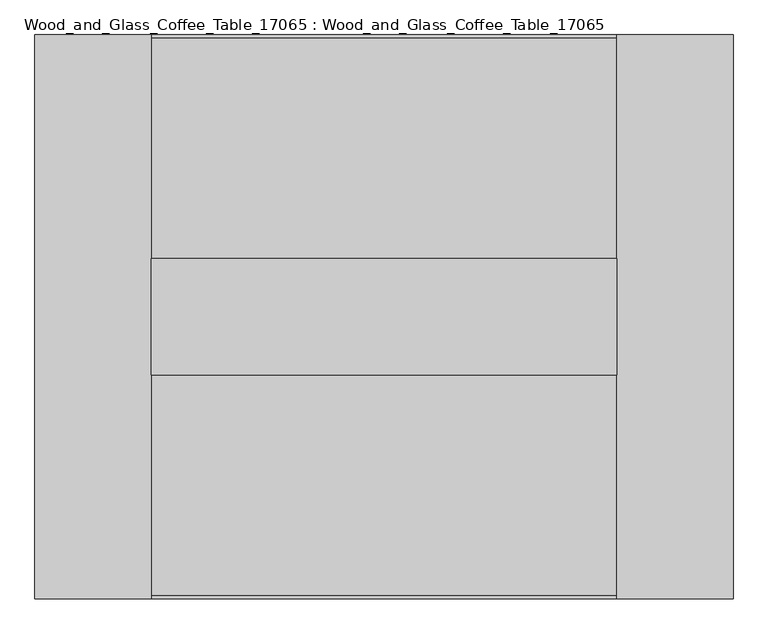
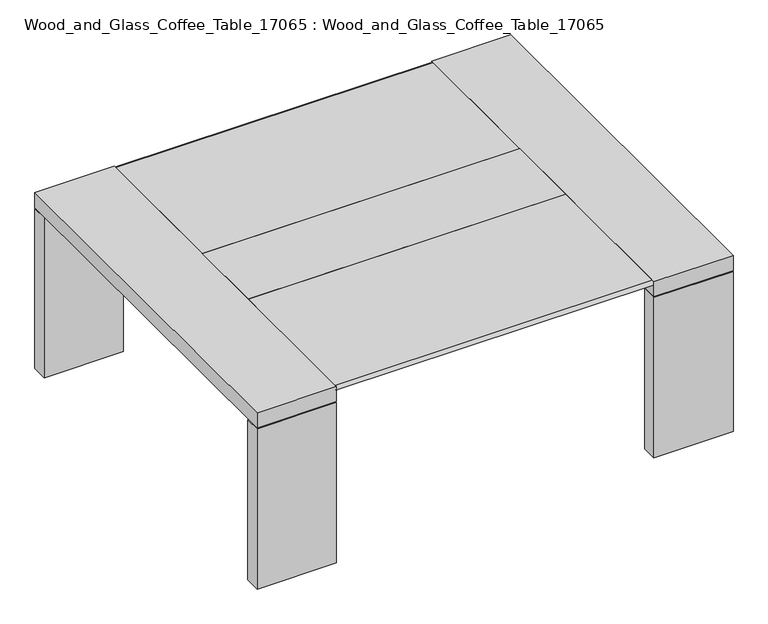
"""IFC4 building model written with IfcOpenShell, lengths in millimetres: furniture geometry, Wood_and_Glass_Coffee_Table_17065 : Wood_and_Glass_Coffee_Table_17065."""

from ifc_helpers import new_model, si_unit, frame, origin, place, context, project, spatial, polyline, circle_curve, outline, extrude, faceted_brep, source, transform, mapped, element, save
from ifc_brep_helpers import plane_surface, cylinder_surface, advanced_brep


def wood_and_glass_coffee_table_17065_wood_and_glass_coffee_dbc724b2(model_context):
    return source(origin(), model_context, "Body", "SolidModel", [
        extrude(outline(polyline([(-400.0, -100.0), (-400.0, 100.0), (400.0, 100.0), (400.0, -100.0), (-400.0, -100.0)])), frame((0.0, 0.0, 430.0), z_axis=(0.0, 0.0, 1.0), x_axis=(1.0, 0.0, 0.0)), (0.0, 0.0, 1.0), 40.0),
        faceted_brep([(-600.0, -484.8341606, 470.0), (-400.0, -484.8341606, 470.0), (-400.0, -478.8341606, 470.0), (-400.0, 478.8341606, 470.0), (-400.0, 484.8341606, 470.0), (-600.0, 484.8341606, 470.0), (-600.0, -484.8341606, 430.0), (-600.0, 484.8341606, 430.0), (-400.0, 484.8341606, 430.0), (-400.0, -484.8341606, 430.0), (-400.0, -484.8341606, 458.0), (-400.0, -484.8341606, 464.0), (-400.0, 484.8341606, 458.0), (-400.0, 484.8341606, 464.0)], [[[0, 1, 2, 3, 4, 5]], [[6, 7, 8, 9]], [[1, 0, 6, 9, 10, 11]], [[9, 8, 12, 13, 4, 3, 2, 1, 11, 10]], [[5, 4, 13, 12, 8, 7]], [[0, 5, 7, 6]]]),
        faceted_brep([(400.0, -484.8341606, 470.0), (600.0, -484.8341606, 470.0), (600.0, 484.8341606, 470.0), (400.0, 484.8341606, 470.0), (400.0, 478.8341606, 470.0), (400.0, -478.8341606, 470.0), (400.0, -484.8341606, 430.0), (400.0, 484.8341606, 430.0), (600.0, 484.8341606, 430.0), (600.0, -484.8341606, 430.0), (400.0, -484.8341606, 464.0), (400.0, -484.8341606, 458.0), (400.0, 484.8341606, 458.0), (400.0, 484.8341606, 464.0)], [[[0, 1, 2, 3, 4, 5]], [[6, 7, 8, 9]], [[1, 0, 10, 11, 6, 9]], [[2, 1, 9, 8]], [[3, 2, 8, 7, 12, 13]], [[7, 6, 11, 10, 0, 5, 4, 3, 13, 12]]]),
        advanced_brep(
        [(-400.0, 100.0, 470.0), (400.0, 100.0, 470.0), (400.0, 478.8341606, 470.0), (-400.0, 478.8341606, 470.0), (400.0, 100.0, 458.0), (-400.0, 100.0, 458.0), (-400.0, 478.8341606, 458.0), (400.0, 478.8341606, 458.0), (-400.0, 484.8341606, 464.0), (400.0, 484.8341606, 464.0)],
        [
            (0, 1),
            (1, 2),
            (2, 3),
            (3, 0),
            (4, 5),
            (5, 6),
            (6, 7),
            (7, 4),
            (5, 0),
            (3, 8, circle_curve(frame((-400.0, 478.8341606, 464.0), z_axis=(-1.0, 0.0, 0.0), x_axis=(0.0, 1.0, 0.0)), 6.0)),
            (8, 6, circle_curve(frame((-400.0, 478.8341606, 464.0), z_axis=(-1.0, 0.0, 0.0), x_axis=(0.0, 1.0, 0.0)), 6.0)),
            (4, 1),
            (7, 9, circle_curve(frame((400.0, 478.8341606, 464.0), z_axis=(1.0, 0.0, 0.0), x_axis=(0.0, 1.0, 0.0)), 6.0)),
            (9, 2, circle_curve(frame((400.0, 478.8341606, 464.0), z_axis=(1.0, 0.0, 0.0), x_axis=(0.0, 1.0, 0.0)), 6.0)),
        ],
        [
            plane_surface(frame((-400.0, 484.8341606, 470.0), z_axis=(0.0, 0.0, 1.0), x_axis=(-1.0, 0.0, 0.0))),
            plane_surface(frame((-400.0, 484.8341606, 458.0), z_axis=(0.0, 0.0, -1.0), x_axis=(1.0, 0.0, 0.0))),
            plane_surface(frame((-400.0, 484.8341606, 470.0), z_axis=(-1.0, 0.0, 0.0), x_axis=(0.0, 0.0, -1.0))),
            plane_surface(frame((-400.0, 100.0, 470.0), z_axis=(0.0, -1.0, 0.0), x_axis=(0.0, 0.0, -1.0))),
            plane_surface(frame((400.0, 100.0, 470.0), z_axis=(1.0, 0.0, 0.0), x_axis=(0.0, 0.0, -1.0))),
            cylinder_surface(frame((-400.0, 478.8341606, 464.0), z_axis=(1.0, 0.0, 0.0), x_axis=(0.0, 1.0, 0.0)), 6.0),
        ],
        [
            (0, [[1, 2, 3, 4]]),
            (1, [[5, 6, 7, 8]]),
            (2, [[9, -4, 10, 11, -6]]),
            (3, [[-1, -9, -5, 12]]),
            (4, [[-12, -8, 13, 14, -2]]),
            (5, [[-3, -14, -13, -7, -11, -10]]),
        ],
    ),
        advanced_brep(
        [(400.0, -100.0, 470.0), (-400.0, -100.0, 470.0), (-400.0, -478.8341606, 470.0), (400.0, -478.8341606, 470.0), (-400.0, -100.0, 458.0), (400.0, -100.0, 458.0), (400.0, -478.8341606, 458.0), (-400.0, -478.8341606, 458.0), (-400.0, -484.8341606, 464.0), (400.0, -484.8341606, 464.0)],
        [
            (0, 1),
            (1, 2),
            (2, 3),
            (3, 0),
            (4, 5),
            (5, 6),
            (6, 7),
            (7, 4),
            (0, 5),
            (4, 1),
            (7, 8, circle_curve(frame((-400.0, -478.8341606, 464.0), z_axis=(-1.0, 0.0, 0.0), x_axis=(0.0, 1.0, 0.0)), 6.0)),
            (8, 2, circle_curve(frame((-400.0, -478.8341606, 464.0), z_axis=(-1.0, 0.0, 0.0), x_axis=(0.0, 1.0, 0.0)), 6.0)),
            (3, 9, circle_curve(frame((400.0, -478.8341606, 464.0), z_axis=(1.0, 0.0, 0.0), x_axis=(0.0, 1.0, 0.0)), 6.0)),
            (9, 6, circle_curve(frame((400.0, -478.8341606, 464.0), z_axis=(1.0, 0.0, 0.0), x_axis=(0.0, 1.0, 0.0)), 6.0)),
        ],
        [
            plane_surface(frame((-400.0, 484.8341606, 470.0), z_axis=(0.0, 0.0, 1.0), x_axis=(-1.0, 0.0, 0.0))),
            plane_surface(frame((-400.0, 484.8341606, 458.0), z_axis=(0.0, 0.0, -1.0), x_axis=(1.0, 0.0, 0.0))),
            plane_surface(frame((400.0, -100.0, 470.0), z_axis=(0.0, 1.0, 0.0), x_axis=(0.0, 0.0, -1.0))),
            plane_surface(frame((-400.0, -100.0, 470.0), z_axis=(-1.0, 0.0, 0.0), x_axis=(0.0, 0.0, -1.0))),
            plane_surface(frame((400.0, -484.8341606, 470.0), z_axis=(1.0, 0.0, 0.0), x_axis=(0.0, 0.0, -1.0))),
            cylinder_surface(frame((-400.0, -478.8341606, 464.0), z_axis=(1.0, 0.0, 0.0), x_axis=(0.0, 1.0, 0.0)), 6.0),
        ],
        [
            (0, [[1, 2, 3, 4]]),
            (1, [[5, 6, 7, 8]]),
            (2, [[-1, 9, -5, 10]]),
            (3, [[-10, -8, 11, 12, -2]]),
            (4, [[-9, -4, 13, 14, -6]]),
            (5, [[-3, -12, -11, -7, -14, -13]]),
        ],
    ),
        faceted_brep([(-402.5, -482.3341606, 430.0), (-402.5, -447.3341606, 430.0), (-597.5, -447.3341606, 430.0), (-597.5, -482.3341606, 430.0), (-400.0, -484.8341606, 0.0), (-600.0, -484.8341606, 0.0), (-600.0, -444.8341606, 0.0), (-400.0, -444.8341606, 0.0), (-400.0, -444.8341606, 427.5), (-400.0, -484.8341606, 427.5), (-600.0, -444.8341606, 427.5), (-600.0, -484.8341606, 427.5), (-402.5, -482.3341606, 427.5), (-402.5, -447.3341606, 427.5), (-597.5, -482.3341606, 427.5), (-597.5, -447.3341606, 427.5)], [[[0, 1, 2, 3]], [[4, 5, 6, 7]], [[4, 7, 8, 9]], [[7, 6, 10, 8]], [[6, 5, 11, 10]], [[5, 4, 9, 11]], [[0, 12, 13, 1]], [[12, 0, 3, 14]], [[14, 3, 2, 15]], [[9, 8, 10, 11], [13, 12, 14, 15]], [[1, 13, 15, 2]]]),
        faceted_brep([(597.5, -482.3341606, 430.0), (597.5, -447.3341606, 430.0), (402.5, -447.3341606, 430.0), (402.5, -482.3341606, 430.0), (400.0, -484.8341606, 0.0), (400.0, -444.8341606, 0.0), (600.0, -444.8341606, 0.0), (600.0, -484.8341606, 0.0), (600.0, -484.8341606, 427.5), (400.0, -484.8341606, 427.5), (600.0, -444.8341606, 427.5), (400.0, -444.8341606, 427.5), (597.5, -482.3341606, 427.5), (597.5, -447.3341606, 427.5), (402.5, -482.3341606, 427.5), (402.5, -447.3341606, 427.5)], [[[0, 1, 2, 3]], [[4, 5, 6, 7]], [[4, 7, 8, 9]], [[7, 6, 10, 8]], [[6, 5, 11, 10]], [[5, 4, 9, 11]], [[0, 12, 13, 1]], [[12, 0, 3, 14]], [[14, 3, 2, 15]], [[9, 8, 10, 11], [13, 12, 14, 15]], [[1, 13, 15, 2]]]),
        faceted_brep([(597.5, 447.3341606, 430.0), (597.5, 482.3341606, 430.0), (402.5, 482.3341606, 430.0), (402.5, 447.3341606, 430.0), (400.0, 484.8341606, 0.0), (600.0, 484.8341606, 0.0), (600.0, 444.8341606, 0.0), (400.0, 444.8341606, 0.0), (400.0, 444.8341606, 427.5), (400.0, 484.8341606, 427.5), (600.0, 444.8341606, 427.5), (600.0, 484.8341606, 427.5), (597.5, 447.3341606, 427.5), (597.5, 482.3341606, 427.5), (402.5, 447.3341606, 427.5), (402.5, 482.3341606, 427.5)], [[[0, 1, 2, 3]], [[4, 5, 6, 7]], [[4, 7, 8, 9]], [[7, 6, 10, 8]], [[6, 5, 11, 10]], [[5, 4, 9, 11]], [[0, 12, 13, 1]], [[12, 0, 3, 14]], [[14, 3, 2, 15]], [[9, 8, 10, 11], [13, 12, 14, 15]], [[1, 13, 15, 2]]]),
        faceted_brep([(-597.5, 444.8341606, 430.0), (-402.5, 444.8341606, 430.0), (-402.5, 482.3341606, 430.0), (-597.5, 482.3341606, 430.0), (-400.0, 484.8341606, 0.0), (-400.0, 444.8341606, 0.0), (-600.0, 444.8341606, 0.0), (-600.0, 484.8341606, 0.0), (-600.0, 484.8341606, 427.5), (-400.0, 484.8341606, 427.5), (-600.0, 444.8341606, 427.5), (-400.0, 444.8341606, 427.5), (-402.5, 444.8341606, 427.5), (-597.5, 444.8341606, 427.5), (-402.5, 482.3341606, 427.5), (-597.5, 482.3341606, 427.5)], [[[0, 1, 2, 3]], [[4, 5, 6, 7]], [[4, 7, 8, 9]], [[7, 6, 10, 8]], [[6, 5, 11, 12, 1, 0, 13, 10]], [[5, 4, 9, 11]], [[12, 14, 2, 1]], [[3, 15, 13, 0]], [[14, 12, 11, 9, 8, 10, 13, 15]], [[2, 14, 15, 3]]]),
    ])


if __name__ == "__main__":
    model = new_model("IFC4")
    model_context = context("Model", 3, world=origin())
    ifc_project = project(units=[si_unit("LENGTHUNIT", "METRE", prefix="MILLI")], contexts=[model_context])
    site = spatial("IfcSite", under=ifc_project)
    building = spatial("IfcBuilding", under=site)
    placement = place(None, origin())
    wood_and_glass_coffee_table_17065_wood_and_glass_coffee_shape = wood_and_glass_coffee_table_17065_wood_and_glass_coffee_dbc724b2(model_context)
    element("IfcFurniture", 1, ObjectType="Wood_and_Glass_Coffee_Table_17065 : Wood_and_Glass_Coffee_Table_17065", at=placement, inside=building, context=model_context, shape_type="MappedRepresentation", body=[
        mapped(wood_and_glass_coffee_table_17065_wood_and_glass_coffee_shape, transform((0.0, 0.0, 0.0), x_axis=(1.0, 0.0, 0.0), y_axis=(0.0, 1.0, 0.0), z_axis=(0.0, 0.0, 1.0))),
    ])
    save(model, "model.ifc")

# Revit data of these elements
# Type "Wood_and_Glass_Coffee_Table_17065 : Wood_and_Glass_Coffee_Table_17065"
#   Coffee Table Wood Width = 0' - 7.87402"
#   Coffee Table Width = 3' - 2.17592"
#   Coffee Table Length = 3' - 11.24409"
#   Wood and Glass Coffee Table - Wood = Wood and Glass Coffee Table - Wood
#   Wood and Glass Coffee Table - Glass = Wood and Glass Coffee Table - Glass
#   Default Elevation = 0
# Element 1 (IfcFurniture, "Wood_and_Glass_Coffee_Table_17065 : Wood_and_Glass_Coffee_Table_17065")
#   Materials on its faces: "Wood and Glass Coffee Table - Wood", "Wood and Glass Coffee Table - Glass"
# Materials
#   "Wood and Glass Coffee Table - Wood": class "Generic", colour RGB 120 120 120, transparency 0, Cost = 0
#   "Wood and Glass Coffee Table - Glass": class "Generic", colour RGB 120 120 120, transparency 0, Cost = 0
